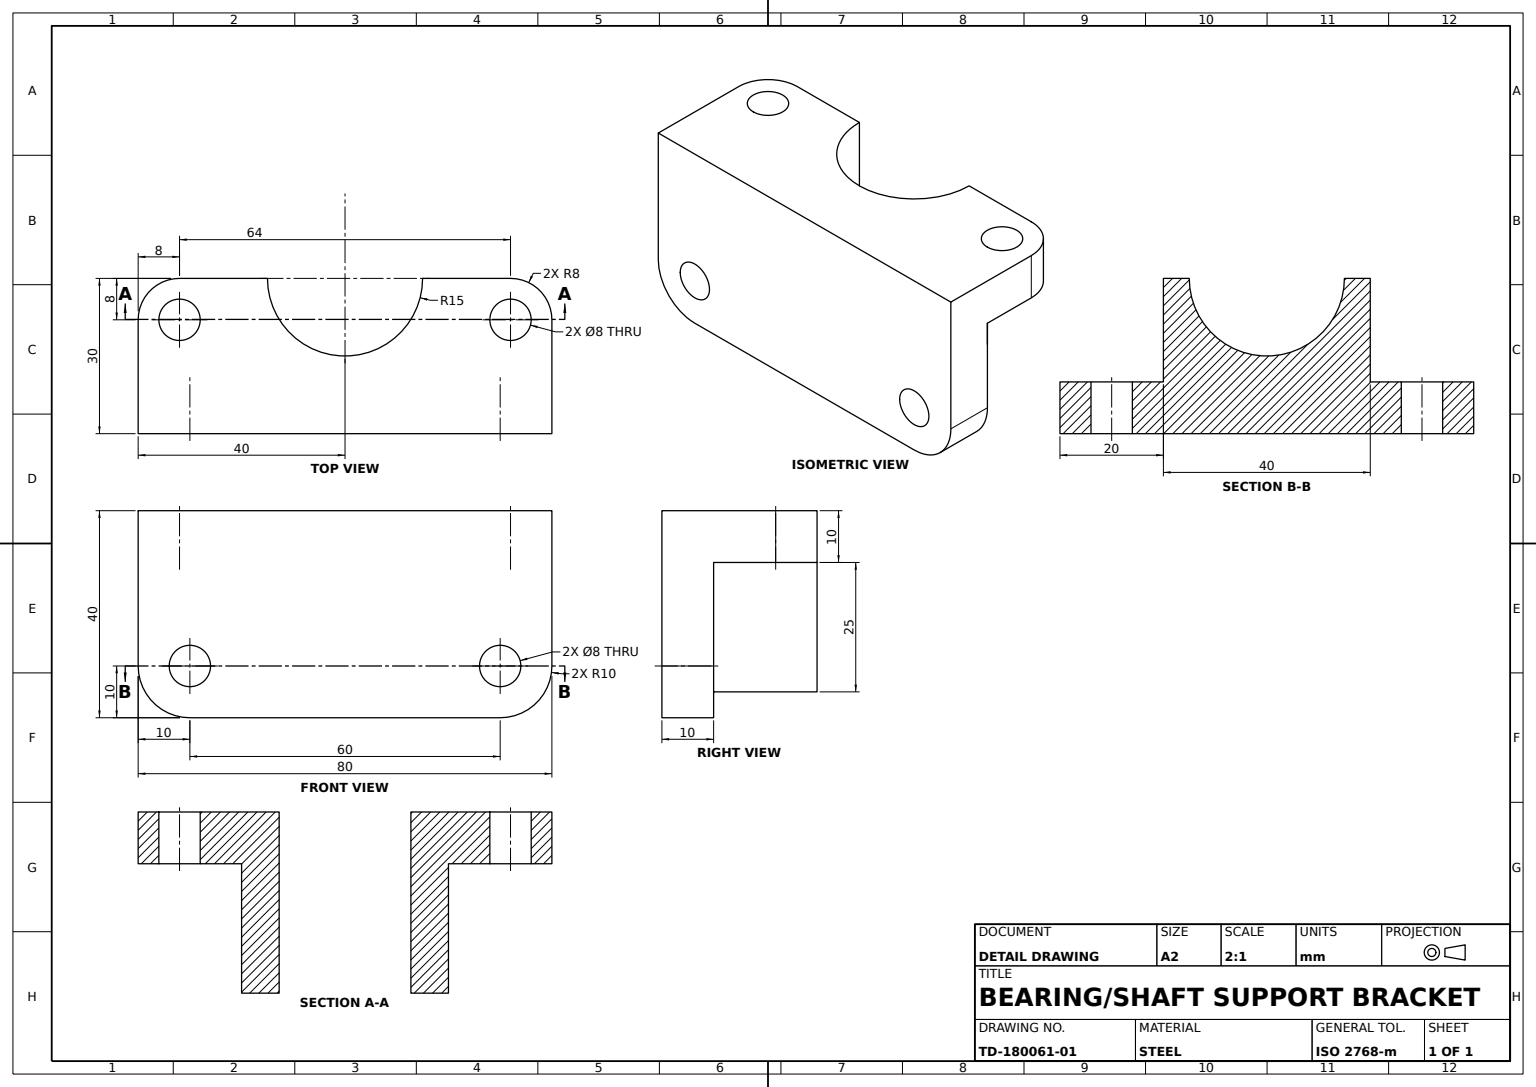
from build123d import *

# Parameters (mm, degrees)
BASE_PLATE_DEPTH              = 10
LUG_FLANGE_DEPTH              = 10
SADDLE_BLOCK_DEPTH            = 25
HALF_ROUND_CRADLE_CUT_DEPTH   = 35
BASE_PLATE_LUG_HOLES_SKETCH_R = 4
BASE_PLATE_LUG_HOLES_2X_DEPTH = 35
FLANGE_LUG_HOLES_SKETCH_R     = 4
FLANGE_LUG_HOLES_2X_DEPTH     = 35


with BuildPart() as part:
    # Base Plate Sketch → Base Plate (new body)
    with BuildSketch(Plane.XY):
        with BuildLine():
            Line((0, 0), (80, 0))
            Line((80, 0), (80, -30))
            ThreePointArc((80, -30), (77.071067812, -37.071067812), (70, -40))
            Line((70, -40), (10, -40))
            ThreePointArc((10, -40), (2.928932188, -37.071067812), (0, -30))
            Line((0, -30), (0, 0))
        make_face()
    extrude(amount=BASE_PLATE_DEPTH)

    # Lug Flange Sketch → Lug Flange (add)
    with BuildSketch(Plane(origin=(0, 0, 0), x_dir=(1, 0, 0), z_dir=(0, 1, 0))):
        with BuildLine():
            Line((8, 20), (72, 20))
            ThreePointArc((72, 20), (77.656854249, 17.656854249), (80, 12))
            Line((80, 12), (80, 0))
            Line((80, 0), (0, 0))
            Line((0, 0), (0, 12))
            ThreePointArc((0, 12), (2.343145751, 17.656854249), (8, 20))
        make_face()
    extrude(amount=-LUG_FLANGE_DEPTH)

    # Saddle Block Sketch → Saddle Block (add)
    with BuildSketch(Plane.XZ.offset(10)):
        Polygon((40, 0), (60, 0), (60, -20), (20, -20), (20, 0), align=None)
    extrude(amount=SADDLE_BLOCK_DEPTH)

    # Cradle Sketch → Half-Round Cradle Cut (cut)
    with BuildSketch(Plane.XZ.offset(35)):
        with BuildLine():
            Line((25, -20), (55, -20))
            ThreePointArc((55, -20), (40, -5), (25, -20))
        make_face()
    extrude(amount=-HALF_ROUND_CRADLE_CUT_DEPTH, mode=Mode.SUBTRACT)

    # Base Plate Lug Holes Sketch → Base Plate Lug Holes 2x (cut)
    with BuildSketch(Plane(origin=(0, 0, 0), x_dir=(-1, 0, 0), z_dir=(0, 0, -1))):
        with Locations((-70, -30)):
            Circle(BASE_PLATE_LUG_HOLES_SKETCH_R)
        with Locations((-10, -30)):
            Circle(BASE_PLATE_LUG_HOLES_SKETCH_R)
    extrude(amount=-BASE_PLATE_LUG_HOLES_2X_DEPTH, mode=Mode.SUBTRACT)

    # Flange Lug Holes Sketch → Flange Lug Holes 2x (cut)
    with BuildSketch(Plane.XZ.offset(10)):
        with Locations(Location((72, -12, 0), (0, 0, 270))):
            Circle(FLANGE_LUG_HOLES_SKETCH_R)
        with Locations(Location((8, -12, 0), (0, 0, 270))):
            Circle(FLANGE_LUG_HOLES_SKETCH_R)
    extrude(amount=-FLANGE_LUG_HOLES_2X_DEPTH, mode=Mode.SUBTRACT)


solid = part.part
